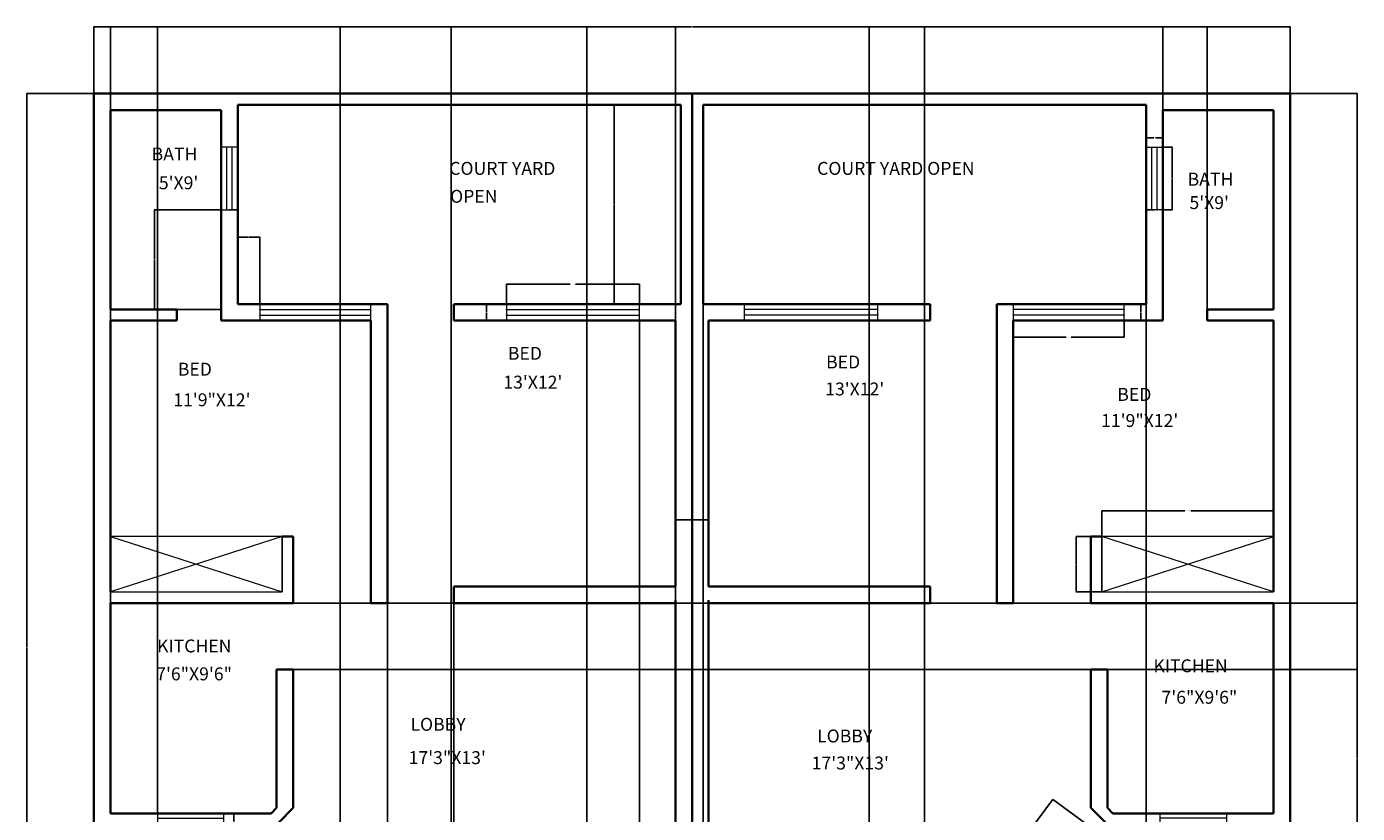
# Model space of a CAD drawing. Units: millimetres. Extents: x 2218 to 2939, y 1369 to 2162.
# Tile 2 of 2: x 2218 to 2939, y 1736 to 2162. Entities that reach past the tile are written whole.
import ezdxf

# ---------------------------------------------------------------- set-up
doc = ezdxf.new("R2010")
doc.units = ezdxf.units.MM
for name, color, linetype, lineweight in [('A-ANNO-DIMS', 2, 'Continuous', 18), ('A-AREA-IDEN', 7, 'Continuous', 25), ('A-FLOR-CASE', 9, 'Continuous', 18), ('A-GLAZ', 4, 'Continuous', 18), ('A-REFR-NODE', 8, 'Continuous', 13), ('A-WALL', 7, 'Continuous', 35)]:
    doc.layers.add(name, color=color, linetype=linetype, lineweight=lineweight)
doc.styles.get("Standard").update_dxf_attribs({"font": 'arial.ttf'})
doc.dimstyles.get("Standard").update_dxf_attribs({"dimtxt": 0.18, "dimasz": 0.18, "dimexe": 0.18, "dimexo": 0.0625, "dimgap": 0.09, "dimtad": 0, "dimtih": 1, "dimtoh": 1, "dimdec": 4, "dimzin": 0, "dimdsep": 46, "dimtxsty": 'Standard', "dimcen": 0.09, "dimadec": 0, "dimazin": 0, "dimtfac": 1, "dimtdec": 4, "dimtofl": 0, "dimtmove": 0, "dimatfit": 3, "dimfxl": 1, "dimtolj": 1, "dimtzin": 0, "dimarcsym": 0})

# ---------------------------------------------------------------- blocks, each defined once
blk = doc.blocks.new('WIN-BATH-COURT')
for p, q in [((9, 34), (0, 34)), ((0, 34), (0, 0)), ((3, 0), (3, 34)), ((6, 0), (6, 34)), ((9, 3), (9, 34)), ((0, 0), (9, 0)), ((9, 0), (4.5, 0))]:
    blk.add_line(p, q)
blk = doc.blocks.new('WIN-BED-OUTER')
for p, q in [((0, 9), (0, 0)), ((60, 0), (60, 9)), ((0, 6), (60, 6)), ((0, 3), (60, 3))]:
    blk.add_line(p, q)
blk = doc.blocks.new('WIN-BED-INNER')
for p, q in [((36, 9), (0, 9)), ((0, 9), (0, 0)), ((72, 0), (72, 9)), ((0, 6), (72, 6)), ((0, 3), (72, 3)), ((0, 0), (72, 0))]:
    blk.add_line(p, q)
blk = doc.blocks.new('WIN-KITCHEN-PORCH')
for p, q in [((18, 9), (0, 9)), ((0, 9), (0, 0)), ((36, 0), (36, 9)), ((0, 6.5), (36, 6.5)), ((0, 2.5), (36, 2.5)), ((0, 0), (36, 0))]:
    blk.add_line(p, q)
blk = doc.blocks.new('CASEWORK-BED')
for p, q in [((93, 30), (0, 30)), ((0, 30), (93, 0)), ((93, 30), (0, 0)), ((93, 30), (93, 0)), ((93, 0), (93, 30)), ((93, 0), (93, 30)), ((0, 0), (93, 0))]:
    blk.add_line(p, q)
blk = doc.blocks.new('*D9')
at = {"layer": 'A-ANNO-DIMS', "color": 0, "lineweight": -2, "transparency": 16777216}
for p, q in [((2833.44, 2096.58), (2838.66, 2096.58)), ((2838.48, 2096.4), (2838.48, 2079.76)), ((2838.48, 2062.76), (2838.48, 2079.39)), ((2833.44, 2062.58), (2838.66, 2062.58))]:
    blk.add_line(p, q, dxfattribs=at)
at = {"layer": 'A-ANNO-DIMS', "color": 0, "transparency": 16777216}
for points in [[(2838.45, 2096.4), (2838.51, 2096.4), (2838.48, 2096.58)], [(2838.45, 2062.76), (2838.51, 2062.76), (2838.48, 2062.58)]]:
    blk.add_solid(points, dxfattribs=at)
at = {"layer": 'Defpoints', "color": 0, "transparency": 16777216}
for p in [(2833.38, 2096.58), (2838.48, 2096.58), (2833.38, 2062.58)]:
    blk.add_point(p, dxfattribs=at)
at = {"layer": 'A-ANNO-DIMS', "color": 0, "transparency": 16777216, "insert": (2838.48, 2079.58), "char_height": 0.18, "attachment_point": 5}
blk.add_mtext('\\A1;BATH WINDOW 34 TYP.', dxfattribs=at)
blk = doc.blocks.new('*D10')
at = {"layer": 'A-ANNO-DIMS', "color": 0, "lineweight": -2, "transparency": 16777216}
for p, q in [((2824.38, 2096.64), (2824.38, 2101.86)), ((2824.56, 2101.68), (2828.42, 2101.68)), ((2833.2, 2101.68), (2829.34, 2101.68)), ((2833.38, 2096.64), (2833.38, 2101.86))]:
    blk.add_line(p, q, dxfattribs=at)
at = {"layer": 'A-ANNO-DIMS', "color": 0, "transparency": 16777216}
for points in [[(2824.56, 2101.71), (2824.56, 2101.65), (2824.38, 2101.68)], [(2833.2, 2101.71), (2833.2, 2101.65), (2833.38, 2101.68)]]:
    blk.add_solid(points, dxfattribs=at)
at = {"layer": 'Defpoints', "color": 0, "transparency": 16777216}
for p in [(2824.38, 2101.68), (2824.38, 2096.58), (2833.38, 2096.58)]:
    blk.add_point(p, dxfattribs=at)
at = {"layer": 'A-ANNO-DIMS', "color": 0, "transparency": 16777216, "insert": (2828.88, 2101.68), "char_height": 0.18, "attachment_point": 5}
blk.add_mtext('\\A1;9 TYP.', dxfattribs=at)
blk = doc.blocks.new('*D11')
at = {"layer": 'A-ANNO-DIMS', "color": 0, "lineweight": -2, "transparency": 16777216}
for p, q in [((2752.38, 2002.51), (2752.38, 1993.4)), ((2812.38, 2002.51), (2812.38, 1993.4)), ((2752.56, 1993.58), (2780.98, 1993.58)), ((2812.2, 1993.58), (2783.78, 1993.58))]:
    blk.add_line(p, q, dxfattribs=at)
at = {"layer": 'A-ANNO-DIMS', "color": 0, "transparency": 16777216}
for points in [[(2752.56, 1993.61), (2752.56, 1993.55), (2752.38, 1993.58)], [(2812.2, 1993.61), (2812.2, 1993.55), (2812.38, 1993.58)]]:
    blk.add_solid(points, dxfattribs=at)
at = {"layer": 'Defpoints', "color": 0, "transparency": 16777216}
for p in [(2752.38, 2002.58), (2812.38, 2002.58), (2752.38, 1993.58)]:
    blk.add_point(p, dxfattribs=at)
at = {"layer": 'A-ANNO-DIMS', "color": 0, "transparency": 16777216, "insert": (2782.38, 1993.58), "char_height": 0.18, "attachment_point": 5}
blk.add_mtext('\\A1;BED WINDOW 60 TYP.', dxfattribs=at)
blk = doc.blocks.new('*D12')
at = {"layer": 'A-ANNO-DIMS', "color": 0, "lineweight": -2, "transparency": 16777216}
for p, q in [((2812.44, 2011.58), (2821.56, 2011.58)), ((2821.38, 2011.4), (2821.38, 2007.26)), ((2821.38, 2002.76), (2821.38, 2006.89)), ((2812.44, 2002.58), (2821.56, 2002.58))]:
    blk.add_line(p, q, dxfattribs=at)
at = {"layer": 'A-ANNO-DIMS', "color": 0, "transparency": 16777216}
for points in [[(2821.35, 2011.4), (2821.41, 2011.4), (2821.38, 2011.58)], [(2821.35, 2002.76), (2821.41, 2002.76), (2821.38, 2002.58)]]:
    blk.add_solid(points, dxfattribs=at)
at = {"layer": 'Defpoints', "color": 0, "transparency": 16777216}
for p in [(2812.38, 2011.58), (2812.38, 2002.58), (2821.38, 2002.58)]:
    blk.add_point(p, dxfattribs=at)
at = {"layer": 'A-ANNO-DIMS', "color": 0, "transparency": 16777216, "insert": (2821.38, 2007.08), "char_height": 0.18, "attachment_point": 5}
blk.add_mtext('\\A1;9 TYP.', dxfattribs=at)
blk = doc.blocks.new('*D13')
at = {"layer": 'A-ANNO-DIMS', "color": 0, "lineweight": -2, "transparency": 16777216}
for p, q in [((2477.88, 2011.64), (2477.88, 2022.56)), ((2478.06, 2022.38), (2512.48, 2022.38)), ((2549.7, 2022.38), (2515.28, 2022.38)), ((2549.88, 2011.64), (2549.88, 2022.56))]:
    blk.add_line(p, q, dxfattribs=at)
at = {"layer": 'A-ANNO-DIMS', "color": 0, "transparency": 16777216}
for points in [[(2478.06, 2022.41), (2478.06, 2022.35), (2477.88, 2022.38)], [(2549.7, 2022.41), (2549.7, 2022.35), (2549.88, 2022.38)]]:
    blk.add_solid(points, dxfattribs=at)
at = {"layer": 'Defpoints', "color": 0, "transparency": 16777216}
for p in [(2549.88, 2022.38), (2477.88, 2011.58), (2549.88, 2011.58)]:
    blk.add_point(p, dxfattribs=at)
at = {"layer": 'A-ANNO-DIMS', "color": 0, "transparency": 16777216, "insert": (2513.88, 2022.38), "char_height": 0.18, "attachment_point": 5}
blk.add_mtext('\\A1;BED WINDOW 72 TYP.', dxfattribs=at)
blk = doc.blocks.new('*D14')
at = {"layer": 'A-ANNO-DIMS', "color": 0, "lineweight": -2, "transparency": 16777216}
for p, q in [((2477.82, 2011.58), (2466.9, 2011.58)), ((2467.08, 2011.4), (2467.08, 2007.26)), ((2467.08, 2002.76), (2467.08, 2006.89)), ((2477.82, 2002.58), (2466.9, 2002.58))]:
    blk.add_line(p, q, dxfattribs=at)
at = {"layer": 'A-ANNO-DIMS', "color": 0, "transparency": 16777216}
for points in [[(2467.05, 2011.4), (2467.11, 2011.4), (2467.08, 2011.58)], [(2467.05, 2002.76), (2467.11, 2002.76), (2467.08, 2002.58)]]:
    blk.add_solid(points, dxfattribs=at)
at = {"layer": 'Defpoints', "color": 0, "transparency": 16777216}
for p in [(2467.08, 2011.58), (2477.88, 2011.58), (2477.88, 2002.58)]:
    blk.add_point(p, dxfattribs=at)
at = {"layer": 'A-ANNO-DIMS', "color": 0, "transparency": 16777216, "insert": (2467.08, 2007.08), "char_height": 0.18, "attachment_point": 5}
blk.add_mtext('\\A1;9 TYP.', dxfattribs=at)
blk = doc.blocks.new('*D16')
at = {"layer": 'A-ANNO-DIMS', "color": 0, "lineweight": -2, "transparency": 16777216}
for p, q in [((2324.94, 1735.58), (2330.46, 1735.58)), ((2330.28, 1735.4), (2330.28, 1731.26)), ((2330.28, 1726.76), (2330.28, 1730.89)), ((2324.94, 1726.58), (2330.46, 1726.58))]:
    blk.add_line(p, q, dxfattribs=at)
at = {"layer": 'A-ANNO-DIMS', "color": 0, "transparency": 16777216}
for points in [[(2330.25, 1735.4), (2330.31, 1735.4), (2330.28, 1735.58)], [(2330.25, 1726.76), (2330.31, 1726.76), (2330.28, 1726.58)]]:
    blk.add_solid(points, dxfattribs=at)
at = {"layer": 'Defpoints', "color": 0, "transparency": 16777216}
for p in [(2324.88, 1735.58), (2330.28, 1735.58), (2324.88, 1726.58)]:
    blk.add_point(p, dxfattribs=at)
at = {"layer": 'A-ANNO-DIMS', "color": 0, "transparency": 16777216, "insert": (2330.28, 1731.08), "char_height": 0.18, "attachment_point": 5}
blk.add_mtext('\\A1;9 TYP.', dxfattribs=at)
blk = doc.blocks.new('*D21')
at = {"layer": 'A-ANNO-DIMS', "color": 0, "lineweight": -2, "transparency": 16777216}
for p, q in [((2800.38, 1885.64), (2800.38, 1899.71)), ((2800.56, 1899.53), (2845.29, 1899.53)), ((2893.2, 1899.53), (2848.47, 1899.53)), ((2893.38, 1885.64), (2893.38, 1899.71))]:
    blk.add_line(p, q, dxfattribs=at)
at = {"layer": 'A-ANNO-DIMS', "color": 0, "transparency": 16777216}
for points in [[(2800.56, 1899.56), (2800.56, 1899.5), (2800.38, 1899.53)], [(2893.2, 1899.56), (2893.2, 1899.5), (2893.38, 1899.53)]]:
    blk.add_solid(points, dxfattribs=at)
at = {"layer": 'Defpoints', "color": 0, "transparency": 16777216}
for p in [(2800.38, 1899.53), (2800.38, 1885.58), (2893.38, 1885.58)]:
    blk.add_point(p, dxfattribs=at)
at = {"layer": 'A-ANNO-DIMS', "color": 0, "transparency": 16777216, "insert": (2846.88, 1899.53), "char_height": 0.18, "attachment_point": 5}
blk.add_mtext('\\A1;BED CASEWORK 93 TYP.', dxfattribs=at)
blk = doc.blocks.new('*D22')
at = {"layer": 'A-ANNO-DIMS', "color": 0, "lineweight": -2, "transparency": 16777216}
for p, q in [((2800.32, 1885.58), (2786.25, 1885.58)), ((2786.43, 1885.4), (2786.43, 1870.76)), ((2786.43, 1855.76), (2786.43, 1870.39)), ((2800.32, 1855.58), (2786.25, 1855.58))]:
    blk.add_line(p, q, dxfattribs=at)
at = {"layer": 'A-ANNO-DIMS', "color": 0, "transparency": 16777216}
for points in [[(2786.4, 1885.4), (2786.46, 1885.4), (2786.43, 1885.58)], [(2786.4, 1855.76), (2786.46, 1855.76), (2786.43, 1855.58)]]:
    blk.add_solid(points, dxfattribs=at)
at = {"layer": 'Defpoints', "color": 0, "transparency": 16777216}
for p in [(2800.38, 1885.58), (2786.43, 1855.58), (2800.38, 1855.58)]:
    blk.add_point(p, dxfattribs=at)
at = {"layer": 'A-ANNO-DIMS', "color": 0, "transparency": 16777216, "insert": (2786.43, 1870.58), "char_height": 0.18, "attachment_point": 5}
blk.add_mtext('\\A1;30 TYP.', dxfattribs=at)
blk = doc.blocks.new('*D25')
at = {"layer": 'A-ANNO-DIMS', "color": 0, "lineweight": -2, "transparency": 16777216}
for p, q in [((2254.38, 2125.64), (2254.38, 2161.91)), ((2254.56, 2161.73), (2578.09, 2161.73)), ((2902.2, 2161.73), (2578.67, 2161.73)), ((2902.38, 2125.64), (2902.38, 2161.91))]:
    blk.add_line(p, q, dxfattribs=at)
at = {"layer": 'A-ANNO-DIMS', "color": 0, "transparency": 16777216}
for points in [[(2254.56, 2161.76), (2254.56, 2161.7), (2254.38, 2161.73)], [(2902.2, 2161.76), (2902.2, 2161.7), (2902.38, 2161.73)]]:
    blk.add_solid(points, dxfattribs=at)
at = {"layer": 'Defpoints', "color": 0, "transparency": 16777216}
for p in [(2902.38, 2161.73), (2254.38, 2125.58), (2902.38, 2125.58)]:
    blk.add_point(p, dxfattribs=at)
at = {"layer": 'A-ANNO-DIMS', "color": 0, "transparency": 16777216, "insert": (2578.38, 2161.73), "char_height": 0.18, "attachment_point": 5}
blk.add_mtext('\\A1;648', dxfattribs=at)
blk = doc.blocks.new('*D27')
at = {"layer": 'A-ANNO-DIMS', "color": 0, "lineweight": -2, "transparency": 16777216}
for p, q in [((2902.44, 2125.58), (2938.71, 2125.58)), ((2938.53, 2125.4), (2938.53, 1765.76)), ((2938.53, 1405.76), (2938.53, 1765.39)), ((2902.44, 1405.58), (2938.71, 1405.58))]:
    blk.add_line(p, q, dxfattribs=at)
at = {"layer": 'A-ANNO-DIMS', "color": 0, "transparency": 16777216}
for points in [[(2938.5, 2125.4), (2938.56, 2125.4), (2938.53, 2125.58)], [(2938.5, 1405.76), (2938.56, 1405.76), (2938.53, 1405.58)]]:
    blk.add_solid(points, dxfattribs=at)
at = {"layer": 'Defpoints', "color": 0, "transparency": 16777216}
for p in [(2902.38, 2125.58), (2938.53, 2125.58), (2902.38, 1405.58)]:
    blk.add_point(p, dxfattribs=at)
at = {"layer": 'A-ANNO-DIMS', "color": 0, "transparency": 16777216, "insert": (2938.53, 1765.58), "char_height": 0.18, "attachment_point": 5}
blk.add_mtext('\\A1;720', dxfattribs=at)
blk = doc.blocks.new('*D28')
at = {"layer": 'A-ANNO-DIMS', "color": 0, "lineweight": -2, "transparency": 16777216}
for p, q in [((2254.32, 2125.58), (2218.05, 2125.58)), ((2218.23, 2125.4), (2218.23, 1825.76)), ((2218.23, 1525.76), (2218.23, 1825.39)), ((2254.32, 1525.58), (2218.05, 1525.58))]:
    blk.add_line(p, q, dxfattribs=at)
at = {"layer": 'A-ANNO-DIMS', "color": 0, "transparency": 16777216}
for points in [[(2218.2, 2125.4), (2218.26, 2125.4), (2218.23, 2125.58)], [(2218.2, 1525.76), (2218.26, 1525.76), (2218.23, 1525.58)]]:
    blk.add_solid(points, dxfattribs=at)
at = {"layer": 'Defpoints', "color": 0, "transparency": 16777216}
for p in [(2218.23, 2125.58), (2254.38, 2125.58), (2254.38, 1525.58)]:
    blk.add_point(p, dxfattribs=at)
at = {"layer": 'A-ANNO-DIMS', "color": 0, "transparency": 16777216, "insert": (2218.23, 1825.58), "char_height": 0.18, "attachment_point": 5}
blk.add_mtext('\\A1;600', dxfattribs=at)
blk = doc.blocks.new('*D29')
at = {"layer": 'A-ANNO-DIMS', "color": 0, "lineweight": -2, "transparency": 16777216}
for p, q in [((2584.38, 2119.51), (2584.38, 1369.25)), ((2824.38, 2119.51), (2824.38, 1369.25)), ((2584.56, 1369.43), (2704.09, 1369.43)), ((2824.2, 1369.43), (2704.67, 1369.43))]:
    blk.add_line(p, q, dxfattribs=at)
at = {"layer": 'A-ANNO-DIMS', "color": 0, "transparency": 16777216}
for points in [[(2584.56, 1369.46), (2584.56, 1369.4), (2584.38, 1369.43)], [(2824.2, 1369.46), (2824.2, 1369.4), (2824.38, 1369.43)]]:
    blk.add_solid(points, dxfattribs=at)
at = {"layer": 'Defpoints', "color": 0, "transparency": 16777216}
for p in [(2584.38, 2119.58), (2824.38, 2119.58), (2824.38, 1369.43)]:
    blk.add_point(p, dxfattribs=at)
at = {"layer": 'A-ANNO-DIMS', "color": 0, "transparency": 16777216, "insert": (2704.38, 1369.43), "char_height": 0.18, "attachment_point": 5}
blk.add_mtext('\\A1;240', dxfattribs=at)
blk = doc.blocks.new('*D30')
at = {"layer": 'A-ANNO-DIMS', "color": 0, "lineweight": -2, "transparency": 16777216}
for p, q in [((2572.32, 2119.58), (2536.05, 2119.58)), ((2536.23, 2119.4), (2536.23, 2065.76)), ((2536.23, 2011.76), (2536.23, 2065.39)), ((2572.32, 2011.58), (2536.05, 2011.58))]:
    blk.add_line(p, q, dxfattribs=at)
at = {"layer": 'A-ANNO-DIMS', "color": 0, "transparency": 16777216}
for points in [[(2536.2, 2119.4), (2536.26, 2119.4), (2536.23, 2119.58)], [(2536.2, 2011.76), (2536.26, 2011.76), (2536.23, 2011.58)]]:
    blk.add_solid(points, dxfattribs=at)
at = {"layer": 'Defpoints', "color": 0, "transparency": 16777216}
for p in [(2536.23, 2119.58), (2572.38, 2119.58), (2572.38, 2011.58)]:
    blk.add_point(p, dxfattribs=at)
at = {"layer": 'A-ANNO-DIMS', "color": 0, "transparency": 16777216, "insert": (2536.23, 2065.58), "char_height": 0.18, "attachment_point": 5}
blk.add_mtext('\\A1;108', dxfattribs=at)
blk = doc.blocks.new('*D31')
at = {"layer": 'A-ANNO-DIMS', "color": 0, "lineweight": -2, "transparency": 16777216}
for p, q in [((2387.88, 1612.64), (2387.88, 2161.91)), ((2388.06, 2161.73), (2417.66, 2161.73)), ((2447.7, 2161.73), (2418.1, 2161.73)), ((2447.88, 1612.64), (2447.88, 2161.91))]:
    blk.add_line(p, q, dxfattribs=at)
at = {"layer": 'A-ANNO-DIMS', "color": 0, "transparency": 16777216}
for points in [[(2388.06, 2161.76), (2388.06, 2161.7), (2387.88, 2161.73)], [(2447.7, 2161.76), (2447.7, 2161.7), (2447.88, 2161.73)]]:
    blk.add_solid(points, dxfattribs=at)
at = {"layer": 'Defpoints', "color": 0, "transparency": 16777216}
for p in [(2447.88, 2161.73), (2387.88, 1612.58), (2447.88, 1612.58)]:
    blk.add_point(p, dxfattribs=at)
at = {"layer": 'A-ANNO-DIMS', "color": 0, "transparency": 16777216, "insert": (2417.88, 2161.73), "char_height": 0.18, "attachment_point": 5}
blk.add_mtext('\\A1;60', dxfattribs=at)
blk = doc.blocks.new('*D33')
at = {"layer": 'A-ANNO-DIMS', "color": 0, "lineweight": -2, "transparency": 16777216}
for p, q in [((2323.32, 2062.58), (2287.05, 2062.58)), ((2287.23, 2062.4), (2287.23, 2035.76)), ((2287.23, 2008.76), (2287.23, 2035.39)), ((2323.32, 2008.58), (2287.05, 2008.58))]:
    blk.add_line(p, q, dxfattribs=at)
at = {"layer": 'A-ANNO-DIMS', "color": 0, "transparency": 16777216}
for points in [[(2287.2, 2062.4), (2287.26, 2062.4), (2287.23, 2062.58)], [(2287.2, 2008.76), (2287.26, 2008.76), (2287.23, 2008.58)]]:
    blk.add_solid(points, dxfattribs=at)
at = {"layer": 'Defpoints', "color": 0, "transparency": 16777216}
for p in [(2287.23, 2062.58), (2323.38, 2062.58), (2323.38, 2008.58)]:
    blk.add_point(p, dxfattribs=at)
at = {"layer": 'A-ANNO-DIMS', "color": 0, "transparency": 16777216, "insert": (2287.23, 2035.58), "char_height": 0.18, "attachment_point": 5}
blk.add_mtext('\\A1;54', dxfattribs=at)
blk = doc.blocks.new('*D34')
at = {"layer": 'A-ANNO-DIMS', "color": 0, "lineweight": -2, "transparency": 16777216}
for p, q in [((2332.38, 2011.64), (2332.38, 2047.91)), ((2332.56, 2047.73), (2338.17, 2047.73)), ((2344.2, 2047.73), (2338.59, 2047.73)), ((2344.38, 2011.64), (2344.38, 2047.91))]:
    blk.add_line(p, q, dxfattribs=at)
at = {"layer": 'A-ANNO-DIMS', "color": 0, "transparency": 16777216}
for points in [[(2332.56, 2047.76), (2332.56, 2047.7), (2332.38, 2047.73)], [(2344.2, 2047.76), (2344.2, 2047.7), (2344.38, 2047.73)]]:
    blk.add_solid(points, dxfattribs=at)
at = {"layer": 'Defpoints', "color": 0, "transparency": 16777216}
for p in [(2344.38, 2047.73), (2332.38, 2011.58), (2344.38, 2011.58)]:
    blk.add_point(p, dxfattribs=at)
at = {"layer": 'A-ANNO-DIMS', "color": 0, "transparency": 16777216, "insert": (2338.38, 2047.73), "char_height": 0.18, "attachment_point": 5}
blk.add_mtext('\\A1;12', dxfattribs=at)
blk = doc.blocks.new('*D35')
at = {"layer": 'A-ANNO-DIMS', "color": 0, "lineweight": -2, "transparency": 16777216}
for p, q in [((2549.88, 2002.51), (2549.88, 1369.25)), ((2569.38, 2002.51), (2569.38, 1369.25)), ((2550.06, 1369.43), (2559.31, 1369.43)), ((2569.2, 1369.43), (2559.95, 1369.43))]:
    blk.add_line(p, q, dxfattribs=at)
at = {"layer": 'A-ANNO-DIMS', "color": 0, "transparency": 16777216}
for points in [[(2550.06, 1369.46), (2550.06, 1369.4), (2549.88, 1369.43)], [(2569.2, 1369.46), (2569.2, 1369.4), (2569.38, 1369.43)]]:
    blk.add_solid(points, dxfattribs=at)
at = {"layer": 'Defpoints', "color": 0, "transparency": 16777216}
for p in [(2549.88, 2002.58), (2569.38, 2002.58), (2569.38, 1369.43)]:
    blk.add_point(p, dxfattribs=at)
at = {"layer": 'A-ANNO-DIMS', "color": 0, "transparency": 16777216, "insert": (2559.63, 1369.43), "char_height": 0.18, "attachment_point": 5}
blk.add_mtext('\\A1;19.5', dxfattribs=at)
blk = doc.blocks.new('*D36')
at = {"layer": 'A-ANNO-DIMS', "color": 0, "lineweight": -2, "transparency": 16777216}
for p, q in [((2263.38, 1735.64), (2263.38, 2161.91)), ((2263.56, 2161.73), (2275.8, 2161.73)), ((2288.7, 2161.73), (2276.46, 2161.73)), ((2288.88, 1735.64), (2288.88, 2161.91))]:
    blk.add_line(p, q, dxfattribs=at)
at = {"layer": 'A-ANNO-DIMS', "color": 0, "transparency": 16777216}
for points in [[(2263.56, 2161.76), (2263.56, 2161.7), (2263.38, 2161.73)], [(2288.7, 2161.76), (2288.7, 2161.7), (2288.88, 2161.73)]]:
    blk.add_solid(points, dxfattribs=at)
at = {"layer": 'Defpoints', "color": 0, "transparency": 16777216}
for p in [(2288.88, 2161.73), (2263.38, 1735.58), (2288.88, 1735.58)]:
    blk.add_point(p, dxfattribs=at)
at = {"layer": 'A-ANNO-DIMS', "color": 0, "transparency": 16777216, "insert": (2276.13, 2161.73), "char_height": 0.18, "attachment_point": 5}
blk.add_mtext('\\A1;25.5', dxfattribs=at)
blk = doc.blocks.new('*D37')
at = {"layer": 'A-ANNO-DIMS', "color": 0, "lineweight": -2, "transparency": 16777216}
for p, q in [((2521.38, 1534.64), (2521.38, 2161.91)), ((2521.56, 2161.73), (2545.16, 2161.73)), ((2569.2, 2161.73), (2545.6, 2161.73)), ((2569.38, 1525.64), (2569.38, 2161.91))]:
    blk.add_line(p, q, dxfattribs=at)
at = {"layer": 'A-ANNO-DIMS', "color": 0, "transparency": 16777216}
for points in [[(2521.56, 2161.76), (2521.56, 2161.7), (2521.38, 2161.73)], [(2569.2, 2161.76), (2569.2, 2161.7), (2569.38, 2161.73)]]:
    blk.add_solid(points, dxfattribs=at)
at = {"layer": 'Defpoints', "color": 0, "transparency": 16777216}
for p in [(2569.38, 2161.73), (2521.38, 1534.58), (2569.38, 1525.58)]:
    blk.add_point(p, dxfattribs=at)
at = {"layer": 'A-ANNO-DIMS', "color": 0, "transparency": 16777216, "insert": (2545.38, 2161.73), "char_height": 0.18, "attachment_point": 5}
blk.add_mtext('\\A1;48', dxfattribs=at)
blk = doc.blocks.new('*D38')
at = {"layer": 'A-ANNO-DIMS', "color": 0, "lineweight": -2, "transparency": 16777216}
for p, q in [((2674.38, 1693.64), (2674.38, 2161.91)), ((2674.56, 2161.73), (2689.16, 2161.73)), ((2704.2, 2161.73), (2689.6, 2161.73)), ((2704.38, 1693.64), (2704.38, 2161.91))]:
    blk.add_line(p, q, dxfattribs=at)
at = {"layer": 'A-ANNO-DIMS', "color": 0, "transparency": 16777216}
for points in [[(2674.56, 2161.76), (2674.56, 2161.7), (2674.38, 2161.73)], [(2704.2, 2161.76), (2704.2, 2161.7), (2704.38, 2161.73)]]:
    blk.add_solid(points, dxfattribs=at)
at = {"layer": 'Defpoints', "color": 0, "transparency": 16777216}
for p in [(2704.38, 2161.73), (2674.38, 1693.58), (2704.38, 1693.58)]:
    blk.add_point(p, dxfattribs=at)
at = {"layer": 'A-ANNO-DIMS', "color": 0, "transparency": 16777216, "insert": (2689.38, 2161.73), "char_height": 0.18, "attachment_point": 5}
blk.add_mtext('\\A1;30', dxfattribs=at)
blk = doc.blocks.new('*D39')
at = {"layer": 'A-ANNO-DIMS', "color": 0, "lineweight": -2, "transparency": 16777216}
for p, q in [((2413.38, 1849.51), (2413.38, 1369.25)), ((2449.38, 1849.51), (2449.38, 1369.25)), ((2413.56, 1369.43), (2431.16, 1369.43)), ((2449.2, 1369.43), (2431.6, 1369.43))]:
    blk.add_line(p, q, dxfattribs=at)
at = {"layer": 'A-ANNO-DIMS', "color": 0, "transparency": 16777216}
for points in [[(2413.56, 1369.46), (2413.56, 1369.4), (2413.38, 1369.43)], [(2449.2, 1369.46), (2449.2, 1369.4), (2449.38, 1369.43)]]:
    blk.add_solid(points, dxfattribs=at)
at = {"layer": 'Defpoints', "color": 0, "transparency": 16777216}
for p in [(2413.38, 1849.58), (2449.38, 1849.58), (2449.38, 1369.43)]:
    blk.add_point(p, dxfattribs=at)
at = {"layer": 'A-ANNO-DIMS', "color": 0, "transparency": 16777216, "insert": (2431.38, 1369.43), "char_height": 0.18, "attachment_point": 5}
blk.add_mtext('\\A1;36', dxfattribs=at)
blk = doc.blocks.new('*D41')
at = {"layer": 'A-ANNO-DIMS', "color": 0, "lineweight": -2, "transparency": 16777216}
for p, q in [((2362.44, 1849.58), (2938.71, 1849.58)), ((2938.53, 1849.4), (2938.53, 1831.76)), ((2938.53, 1813.76), (2938.53, 1831.39)), ((2362.44, 1813.58), (2938.71, 1813.58))]:
    blk.add_line(p, q, dxfattribs=at)
at = {"layer": 'A-ANNO-DIMS', "color": 0, "transparency": 16777216}
for points in [[(2938.5, 1849.4), (2938.56, 1849.4), (2938.53, 1849.58)], [(2938.5, 1813.76), (2938.56, 1813.76), (2938.53, 1813.58)]]:
    blk.add_solid(points, dxfattribs=at)
at = {"layer": 'Defpoints', "color": 0, "transparency": 16777216}
for p in [(2362.38, 1849.58), (2938.53, 1849.58), (2362.38, 1813.58)]:
    blk.add_point(p, dxfattribs=at)
at = {"layer": 'A-ANNO-DIMS', "color": 0, "transparency": 16777216, "insert": (2938.53, 1831.58), "char_height": 0.18, "attachment_point": 5}
blk.add_mtext('\\A1;36', dxfattribs=at)
blk = doc.blocks.new('*D42')
at = {"layer": 'A-ANNO-DIMS', "color": 0, "lineweight": -2, "transparency": 16777216}
for p, q in [((2833.38, 2008.64), (2833.38, 2161.91)), ((2833.56, 2161.73), (2845.16, 2161.73)), ((2857.2, 2161.73), (2845.6, 2161.73)), ((2857.38, 2008.64), (2857.38, 2161.91))]:
    blk.add_line(p, q, dxfattribs=at)
at = {"layer": 'A-ANNO-DIMS', "color": 0, "transparency": 16777216}
for points in [[(2833.56, 2161.76), (2833.56, 2161.7), (2833.38, 2161.73)], [(2857.2, 2161.76), (2857.2, 2161.7), (2857.38, 2161.73)]]:
    blk.add_solid(points, dxfattribs=at)
at = {"layer": 'Defpoints', "color": 0, "transparency": 16777216}
for p in [(2857.38, 2161.73), (2833.38, 2008.58), (2857.38, 2008.58)]:
    blk.add_point(p, dxfattribs=at)
at = {"layer": 'A-ANNO-DIMS', "color": 0, "transparency": 16777216, "insert": (2845.38, 2161.73), "char_height": 0.18, "attachment_point": 5}
blk.add_mtext('\\A1;24', dxfattribs=at)
blk = doc.blocks.new('*D43')
at = {"layer": 'A-ANNO-DIMS', "color": 0, "lineweight": -2, "transparency": 16777216}
for p, q in [((2569.38, 1858.64), (2569.38, 1894.91)), ((2569.56, 1894.73), (2578.17, 1894.73)), ((2587.2, 1894.73), (2578.59, 1894.73)), ((2587.38, 1858.64), (2587.38, 1894.91))]:
    blk.add_line(p, q, dxfattribs=at)
at = {"layer": 'A-ANNO-DIMS', "color": 0, "transparency": 16777216}
for points in [[(2569.56, 1894.76), (2569.56, 1894.7), (2569.38, 1894.73)], [(2587.2, 1894.76), (2587.2, 1894.7), (2587.38, 1894.73)]]:
    blk.add_solid(points, dxfattribs=at)
at = {"layer": 'Defpoints', "color": 0, "transparency": 16777216}
for p in [(2587.38, 1894.73), (2569.38, 1858.58), (2587.38, 1858.58)]:
    blk.add_point(p, dxfattribs=at)
at = {"layer": 'A-ANNO-DIMS', "color": 0, "transparency": 16777216, "insert": (2578.38, 1894.73), "char_height": 0.18, "attachment_point": 5}
blk.add_mtext('\\A1;18', dxfattribs=at)
blk = doc.blocks.new('*D44')
at = {"layer": 'A-ANNO-DIMS', "color": 0, "lineweight": -2, "transparency": 16777216}
for p, q in [((2773.57, 1742.97), (2761.75, 1726.84)), ((2802.78, 1721.77), (2773.53, 1743.22)), ((2749.66, 1710.36), (2761.48, 1726.48)), ((2778.65, 1688.87), (2749.4, 1710.32))]:
    blk.add_line(p, q, dxfattribs=at)
at = {"layer": 'A-ANNO-DIMS', "color": 0, "transparency": 16777216}
for points in [[(2773.55, 1742.99), (2773.6, 1742.95), (2773.68, 1743.11)], [(2749.63, 1710.37), (2749.68, 1710.34), (2749.55, 1710.21)]]:
    blk.add_solid(points, dxfattribs=at)
at = {"layer": 'Defpoints', "color": 0, "transparency": 16777216}
for p in [(2773.68, 1743.11), (2802.83, 1721.74), (2778.7, 1688.83)]:
    blk.add_point(p, dxfattribs=at)
at = {"layer": 'A-ANNO-DIMS', "color": 0, "transparency": 16777216, "insert": (2761.61, 1726.66), "char_height": 0.18, "attachment_point": 5}
blk.add_mtext('\\A1;40.8', dxfattribs=at)

msp = doc.modelspace()

# ---------------------------------------------------------------- linework, layer by layer
at = {"layer": 'A-REFR-NODE'}
for p in [(2326.38, 2062.58), (2329.38, 2062.58), (2827.38, 2062.58), (2830.38, 2062.58), (2344.38, 2008.58), (2344.38, 2005.58), (2477.88, 2008.58), (2477.88, 2005.58), (2678.88, 2008.58), (2678.88, 2005.58), (2812.38, 2008.58), (2812.38, 2005.58)]:
    msp.add_point(p, dxfattribs=at)
at = {"layer": 'A-WALL'}
for p, q in [((2254.38, 2125.58), (2578.38, 2125.58)), ((2254.38, 2125.58), (2254.38, 1525.58)), ((2572.38, 2119.58), (2332.38, 2119.58)), ((2332.38, 2119.58), (2332.38, 2011.58)), ((2578.38, 2125.58), (2572.38, 2125.58)), ((2572.38, 2011.58), (2572.38, 2119.58)), ((2578.38, 2125.58), (2578.38, 1525.58)), ((2902.38, 2125.58), (2578.38, 2125.58)), ((2578.38, 2125.58), (2578.38, 1525.58)), ((2578.38, 2125.58), (2584.38, 2125.58)), ((2584.38, 2119.58), (2824.38, 2119.58)), ((2584.38, 2011.58), (2584.38, 2119.58)), ((2824.38, 2119.58), (2824.38, 2011.58)), ((2902.38, 2125.58), (2902.38, 1525.58)), ((2263.38, 2116.58), (2323.38, 2116.58)), ((2263.38, 2008.58), (2263.38, 2116.58)), ((2263.38, 2116.58), (2263.38, 2008.58)), ((2263.38, 2116.58), (2263.38, 2008.58)), ((2323.38, 2116.58), (2323.38, 2008.58)), ((2893.38, 2116.58), (2833.38, 2116.58)), ((2833.38, 2116.58), (2833.38, 2008.58)), ((2893.38, 2008.58), (2893.38, 2116.58)), ((2893.38, 2116.58), (2893.38, 2008.58)), ((2893.38, 2116.58), (2893.38, 2008.58)), ((2332.38, 2011.58), (2332.38, 2065.58)), ((2824.38, 2011.58), (2824.38, 2065.58)), ((2332.38, 2011.58), (2413.38, 2011.58)), ((2332.38, 2011.58), (2344.38, 2011.58)), ((2413.38, 2002.58), (2413.38, 2011.58)), ((2449.38, 2011.58), (2449.38, 2002.58)), ((2449.38, 2011.58), (2572.38, 2011.58)), ((2707.38, 2011.58), (2584.38, 2011.58)), ((2707.38, 2011.58), (2707.38, 2002.58)), ((2824.38, 2011.58), (2743.38, 2011.58)), ((2743.38, 2002.58), (2743.38, 2011.58)), ((2824.38, 2011.58), (2812.38, 2011.58)), ((2299.38, 2008.58), (2263.38, 2008.58)), ((2299.38, 2002.58), (2299.38, 2008.58)), ((2323.38, 2004.08), (2323.38, 2008.58)), ((2323.38, 2002.58), (2323.38, 2008.58)), ((2833.38, 2004.08), (2833.38, 2008.58)), ((2833.38, 2002.58), (2833.38, 2008.58)), ((2857.38, 2008.58), (2893.38, 2008.58)), ((2857.38, 2002.58), (2857.38, 2008.58)), ((2263.38, 2002.58), (2263.38, 1860.08)), ((2263.38, 2002.58), (2299.38, 2002.58)), ((2323.38, 2002.58), (2404.38, 2002.58)), ((2404.38, 1860.08), (2404.38, 2002.58)), ((2413.38, 2002.58), (2413.38, 1860.08)), ((2413.38, 2002.58), (2413.38, 1860.08)), ((2449.38, 2002.58), (2569.38, 2002.58)), ((2449.38, 2002.58), (2569.38, 2002.58)), ((2569.38, 2002.58), (2513.88, 2002.58)), ((2569.38, 1860.08), (2569.38, 2002.58)), ((2569.38, 2002.58), (2569.38, 1858.58)), ((2587.38, 1860.08), (2587.38, 2002.58)), ((2707.38, 2002.58), (2587.38, 2002.58)), ((2587.38, 2002.58), (2587.38, 1858.58)), ((2707.38, 2002.58), (2587.38, 2002.58)), ((2587.38, 2002.58), (2642.88, 2002.58)), ((2743.38, 2002.58), (2743.38, 1860.08)), ((2743.38, 2002.58), (2743.38, 1860.08)), ((2752.38, 1860.08), (2752.38, 2002.58)), ((2833.38, 2002.58), (2752.38, 2002.58)), ((2893.38, 2002.58), (2857.38, 2002.58)), ((2893.38, 2002.58), (2893.38, 1860.08)), ((2362.38, 1885.58), (2356.38, 1885.58)), ((2362.38, 1855.58), (2362.38, 1885.58)), ((2794.38, 1855.58), (2794.38, 1885.58)), ((2794.38, 1885.58), (2800.38, 1885.58)), ((2263.38, 1860.08), (2263.38, 1855.58)), ((2404.38, 1854.08), (2404.38, 1860.08)), ((2413.38, 1849.58), (2413.38, 1860.08)), ((2569.38, 1860.08), (2569.38, 1858.58)), ((2587.38, 1860.08), (2587.38, 1858.58)), ((2743.38, 1849.58), (2743.38, 1860.08)), ((2752.38, 1854.08), (2752.38, 1860.08)), ((2893.38, 1860.08), (2893.38, 1855.58)), ((2362.38, 1849.58), (2362.38, 1855.58)), ((2404.38, 1855.58), (2404.38, 1849.58)), ((2413.38, 1858.58), (2413.38, 1849.58)), ((2569.38, 1858.58), (2449.38, 1858.58)), ((2449.38, 1858.58), (2449.38, 1849.58)), ((2587.38, 1858.58), (2707.38, 1858.58)), ((2707.38, 1858.58), (2707.38, 1849.58)), ((2743.38, 1858.58), (2743.38, 1849.58)), ((2752.38, 1855.58), (2752.38, 1849.58)), ((2794.38, 1849.58), (2794.38, 1855.58)), ((2353.38, 1849.58), (2263.38, 1849.58)), ((2263.38, 1849.58), (2263.38, 1735.58)), ((2263.38, 1735.58), (2263.38, 1849.58)), ((2353.38, 1849.58), (2362.38, 1849.58)), ((2404.38, 1849.58), (2413.38, 1849.58)), ((2413.38, 1849.58), (2404.38, 1849.58)), ((2449.38, 1849.58), (2569.38, 1849.58)), ((2569.38, 1849.58), (2449.38, 1849.58)), ((2569.38, 1695.08), (2569.38, 1851.08)), ((2587.38, 1695.08), (2587.38, 1851.08)), ((2707.38, 1849.58), (2587.38, 1849.58)), ((2587.38, 1849.58), (2707.38, 1849.58)), ((2752.38, 1849.58), (2743.38, 1849.58)), ((2743.38, 1849.58), (2752.38, 1849.58)), ((2803.38, 1849.58), (2794.38, 1849.58)), ((2803.38, 1849.58), (2893.38, 1849.58)), ((2893.38, 1849.58), (2893.38, 1735.58)), ((2893.38, 1735.58), (2893.38, 1849.58)), ((2353.38, 1738.58), (2353.38, 1813.58)), ((2362.38, 1813.58), (2353.38, 1813.58)), ((2362.38, 1813.58), (2362.38, 1738.58)), ((2362.38, 1813.58), (2362.38, 1738.58)), ((2794.38, 1813.58), (2794.38, 1738.58)), ((2794.38, 1813.58), (2794.38, 1738.58)), ((2794.38, 1813.58), (2803.38, 1813.58)), ((2803.38, 1738.58), (2803.38, 1813.58)), ((2350.38, 1735.58), (2353.38, 1738.58)), ((2354.53, 1730.72), (2362.38, 1738.58)), ((2802.23, 1730.72), (2794.38, 1738.58)), ((2806.38, 1735.58), (2803.38, 1738.58)), ((2263.38, 1735.58), (2350.38, 1735.58)), ((2893.38, 1735.58), (2806.38, 1735.58))]:
    msp.add_line(p, q, dxfattribs=at)

# ---------------------------------------------------------------- block references
at = {"layer": 'A-FLOR-CASE'}
msp.add_blockref('CASEWORK-BED', (2263.38, 1855.58), dxfattribs=at)
at = {"layer": 'A-FLOR-CASE', "rotation": 180}
msp.add_blockref('CASEWORK-BED', (2893.38, 1885.58), dxfattribs=at)
at = {"layer": 'A-GLAZ'}
for name, p in [('WIN-BATH-COURT', (2323.38, 2062.58)), ('WIN-BED-OUTER', (2344.38, 2002.58)), ('WIN-BED-INNER', (2477.88, 2002.58)), ('WIN-KITCHEN-PORCH', (2288.88, 1726.58))]:
    msp.add_blockref(name, p, dxfattribs=at)
at = {"layer": 'A-GLAZ', "extrusion": (0, 0, -1), "zscale": -1}
for name, p in [('WIN-BATH-COURT', (-2833.38, 2062.58)), ('WIN-BED-INNER', (-2678.88, 2002.58)), ('WIN-KITCHEN-PORCH', (-2867.88, 1726.58))]:
    msp.add_blockref(name, p, dxfattribs=at)
at = {"layer": 'A-GLAZ', "rotation": 180}
msp.add_blockref('WIN-BED-OUTER', (2812.38, 2011.58), dxfattribs=at)

# ---------------------------------------------------------------- texts
at = {"layer": 'A-ANNO-DIMS'}
for s, p in [("5'X9'", (2289.65, 2073.77)), ("5'X9'", (2847.79, 2063.04)), ("13'X12'", (2476.2, 1965.75)), ("13'X12'", (2650.51, 1962.04)), ('11\'9"X12\'', (2297.46, 1956.18)), ('11\'9"X12\'', (2799.94, 1944.96)), ('7\'6"X9\'6"', (2288.2, 1807.67)), ('7\'6"X9\'6"', (2832.67, 1794.99)), ('17\'3"X13\'', (2424.93, 1762.3)), ('17\'3"X13\'', (2643.2, 1759.37))]:
    msp.add_text(s, height=7, dxfattribs=at).set_placement(p)
at = {"layer": 'A-AREA-IDEN'}
for s, p in [('BATH', (2285.74, 2089.38)), ('COURT YARD ', (2446.89, 2081.58)), ('COURT YARD OPEN', (2646.12, 2081.58)), ('BATH', (2846.81, 2075.72)), ('OPEN', (2447.38, 2066.45)), ('BED', (2478.64, 1981.37)), ('BED', (2651, 1976.68)), ('BED', (2299.91, 1972.77)), ('BED', (2808.72, 1959.11)), ('KITCHEN', (2288.69, 1822.8)), ('KITCHEN', (2828.27, 1812.06)), ('LOBBY', (2425.9, 1780.35)), ('LOBBY', (2646.13, 1774.01))]:
    msp.add_text(s, height=7, dxfattribs=at).set_placement(p)

# ---------------------------------------------------------------- dimensions: what is measured, and where the dimension line sits
at = {"layer": 'A-ANNO-DIMS'}
for base, p1, p2, override, picture, middle in [((2902.38, 2161.73), (2254.38, 2125.58), (2902.38, 2125.58), {"dimdec": 0, "dimlfac": 1, "dimrnd": 0, "dimzin": 0, "dimdsep": 46, "dimlunit": 2}, '*D25', (2578.38, 2161.73)), ((2288.88, 2161.73), (2263.38, 1735.58), (2288.88, 1735.58), {"dimdec": 1, "dimlfac": 1, "dimrnd": 0, "dimzin": 0, "dimdsep": 46, "dimlunit": 2}, '*D36', (2276.13, 2161.73)), ((2447.88, 2161.73), (2387.88, 1612.58), (2447.88, 1612.58), {"dimdec": 0, "dimlfac": 1, "dimrnd": 0, "dimzin": 0, "dimdsep": 46, "dimlunit": 2}, '*D31', (2417.88, 2161.73)), ((2569.38, 2161.73), (2521.38, 1534.58), (2569.38, 1525.58), {"dimdec": 0, "dimlfac": 1, "dimrnd": 0, "dimzin": 0, "dimdsep": 46, "dimlunit": 2}, '*D37', (2545.38, 2161.73)), ((2704.38, 2161.73), (2674.38, 1693.58), (2704.38, 1693.58), {"dimdec": 0, "dimlfac": 1, "dimrnd": 0, "dimzin": 0, "dimdsep": 46, "dimlunit": 2}, '*D38', (2689.38, 2161.73)), ((2857.38, 2161.73), (2833.38, 2008.58), (2857.38, 2008.58), {"dimdec": 0, "dimlfac": 1, "dimrnd": 0, "dimzin": 0, "dimdsep": 46, "dimlunit": 2}, '*D42', (2845.38, 2161.73)), ((2824.38, 1369.43), (2584.38, 2119.58), (2824.38, 2119.58), {"dimdec": 0, "dimlfac": 1, "dimrnd": 0, "dimzin": 0, "dimdsep": 46, "dimlunit": 2}, '*D29', (2704.38, 1369.43)), ((2344.38, 2047.73), (2332.38, 2011.58), (2344.38, 2011.58), {"dimdec": 0, "dimlfac": 1, "dimrnd": 0, "dimzin": 0, "dimdsep": 46, "dimlunit": 2}, '*D34', (2338.38, 2047.73)), ((2569.38, 1369.43), (2549.88, 2002.58), (2569.38, 2002.58), {"dimdec": 1, "dimlfac": 1, "dimrnd": 0, "dimzin": 0, "dimdsep": 46, "dimlunit": 2}, '*D35', (2559.63, 1369.43)), ((2587.38, 1894.73), (2569.38, 1858.58), (2587.38, 1858.58), {"dimdec": 0, "dimlfac": 1, "dimrnd": 0, "dimzin": 0, "dimdsep": 46, "dimlunit": 2}, '*D43', (2578.38, 1894.73)), ((2449.38, 1369.43), (2413.38, 1849.58), (2449.38, 1849.58), {"dimdec": 0, "dimlfac": 1, "dimrnd": 0, "dimzin": 0, "dimdsep": 46, "dimlunit": 2}, '*D39', (2431.38, 1369.43))]:
    dim = msp.add_linear_dim(base=base, p1=p1, p2=p2, dimstyle='Standard', override=override, dxfattribs=at)
    dim.commit()
    dim.dimension.update_dxf_attribs({"geometry": picture, "text_midpoint": middle})
for base, p1, p2, angle, override, picture, middle in [((2218.23, 2125.58), (2254.38, 1525.58), (2254.38, 2125.58), 90, {"dimdec": 0, "dimlfac": 1, "dimrnd": 0, "dimzin": 0, "dimdsep": 46, "dimlunit": 2}, '*D28', (2218.23, 1825.58)), ((2536.23, 2119.58), (2572.38, 2011.58), (2572.38, 2119.58), 90, {"dimdec": 0, "dimlfac": 1, "dimrnd": 0, "dimzin": 0, "dimdsep": 46, "dimlunit": 2}, '*D30', (2536.23, 2065.58)), ((2938.53, 2125.58), (2902.38, 1405.58), (2902.38, 2125.58), 90, {"dimdec": 0, "dimlfac": 1, "dimrnd": 0, "dimzin": 0, "dimdsep": 46, "dimlunit": 2}, '*D27', (2938.53, 1765.58)), ((2287.23, 2062.58), (2323.38, 2008.58), (2323.38, 2062.58), 90, {"dimdec": 0, "dimlfac": 1, "dimrnd": 0, "dimzin": 0, "dimdsep": 46, "dimlunit": 2}, '*D33', (2287.23, 2035.58)), ((2938.53, 1849.58), (2362.38, 1813.58), (2362.38, 1849.58), 90, {"dimdec": 0, "dimlfac": 1, "dimrnd": 0, "dimzin": 0, "dimdsep": 46, "dimlunit": 2}, '*D41', (2938.53, 1831.58)), ((2773.68, 1743.11), (2778.7, 1688.83), (2802.83, 1721.74), 53.74616, {"dimdec": 1, "dimlfac": 1, "dimrnd": 0, "dimzin": 0, "dimdsep": 46, "dimlunit": 2}, '*D44', (2761.61, 1726.66))]:
    dim = msp.add_linear_dim(base=base, p1=p1, p2=p2, angle=angle, dimstyle='Standard', override=override, dxfattribs=at)
    dim.commit()
    dim.dimension.update_dxf_attribs({"geometry": picture, "text_midpoint": middle})
for base, p1, p2, angle, text, picture, middle in [((2824.38, 2101.68), (2833.38, 2096.58), (2824.38, 2096.58), 180, '<> TYP.', '*D10', (2828.88, 2101.68)), ((2838.48, 2096.58), (2833.38, 2062.58), (2833.38, 2096.58), 90, 'BATH WINDOW <> TYP.', '*D9', (2838.48, 2079.58)), ((2467.08, 2011.58), (2477.88, 2002.58), (2477.88, 2011.58), 90, '<> TYP.', '*D14', (2467.08, 2007.08)), ((2821.38, 2002.58), (2812.38, 2011.58), (2812.38, 2002.58), 270, '<> TYP.', '*D12', (2821.38, 2007.08)), ((2752.38, 1993.58), (2812.38, 2002.58), (2752.38, 2002.58), 180, 'BED WINDOW <> TYP.', '*D11', (2782.38, 1993.58)), ((2800.38, 1899.53), (2893.38, 1885.58), (2800.38, 1885.58), 180, 'BED CASEWORK <> TYP.', '*D21', (2846.88, 1899.53)), ((2786.43, 1855.58), (2800.38, 1885.58), (2800.38, 1855.58), 270, '<> TYP.', '*D22', (2786.43, 1870.58)), ((2330.28, 1735.58), (2324.88, 1726.58), (2324.88, 1735.58), 90, '<> TYP.', '*D16', (2330.28, 1731.08))]:
    dim = msp.add_linear_dim(base=base, p1=p1, p2=p2, angle=angle, text=text, dimstyle='Standard', override={"dimdec": 0, "dimlfac": 1, "dimrnd": 0, "dimzin": 0, "dimdsep": 46, "dimlunit": 2}, dxfattribs=at)
    dim.commit()
    dim.dimension.update_dxf_attribs({"geometry": picture, "text_midpoint": middle})
dim = msp.add_linear_dim(base=(2549.88, 2022.38), p1=(2477.88, 2011.58), p2=(2549.88, 2011.58), text='BED WINDOW <> TYP.', dimstyle='Standard', override={"dimdec": 0, "dimlfac": 1, "dimrnd": 0, "dimzin": 0, "dimdsep": 46, "dimlunit": 2}, dxfattribs=at)
dim.commit()
dim.dimension.update_dxf_attribs({"geometry": '*D13', "text_midpoint": (2513.88, 2022.38)})

doc.saveas('drawing.dxf')
